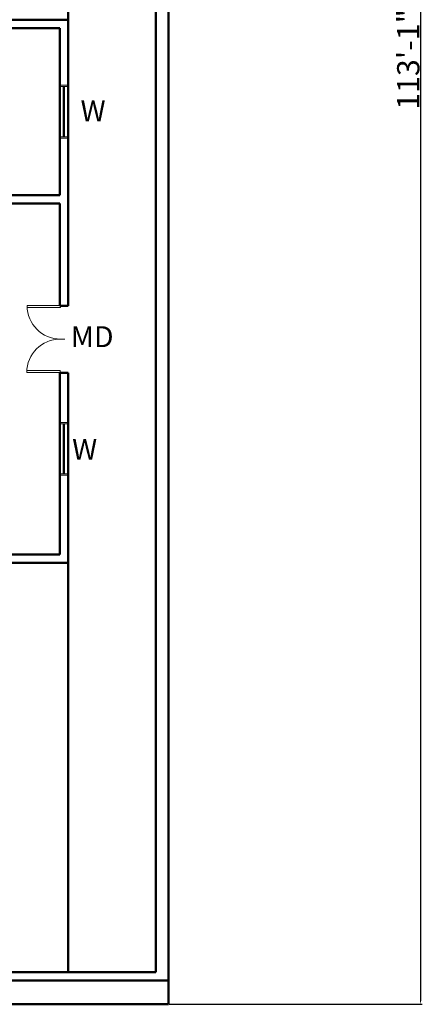
# Model space of a CAD drawing. Units: inches. Extents: x -7040 to -4088, y 6092 to 7645.
# Tile 5 of 11: x -6510 to -6221, y 6157 to 6864. Entities that reach past the tile are written whole.
import ezdxf

# ---------------------------------------------------------------- set-up
doc = ezdxf.new("R2010")
doc.units = ezdxf.units.IN
for name, color, linetype, lineweight in [('A-ANNO-DIMS', 2, 'Continuous', 18), ('A-ANNO-TEXT', 7, 'Continuous', 25), ('A-DOOR', 3, 'Continuous', 18), ('A-GLAZ', 4, 'Continuous', 18), ('A-WALL', 7, 'Continuous', 50)]:
    doc.layers.add(name, color=color, linetype=linetype, lineweight=lineweight)
doc.styles.get("Standard").update_dxf_attribs({"font": 'arial.ttf'})
doc.dimstyles.new('ISO-25', dxfattribs={"dimtxt": 2.5, "dimasz": 2.5, "dimexe": 1.25, "dimexo": 0.625, "dimtad": 1, "dimdec": 0, "dimlunit": 3, "dimtxsty": 'Standard', "dimcen": 2.5, "dimadec": 0, "dimazin": 0, "dimtfac": 1, "dimtdec": 0, "dimtmove": 0, "dimatfit": 3, "dimfxl": 1, "dimarcsym": 0})

# ---------------------------------------------------------------- blocks, each defined once
blk = doc.blocks.new('*U8')
for p, q in [((0, 0), (0, -100)), ((750, 0), (750, -100))]:
    blk.add_line(p, q)
blk.add_lwpolyline([(0, 0), (0, 750), (43.75, 750), (43.75, 0)], close=True)
blk.add_arc((0, 0), 750, 0, 90)
blk = doc.blocks.new('*D93')
at = {"layer": 'A-ANNO-DIMS', "color": 0, "lineweight": -2, "transparency": 16777216}
for p, q in [((-6402.41, 7513.76), (-6220.88, 7513.76)), ((-6222.13, 7511.26), (-6222.13, 6159.26)), ((-6402.41, 6156.76), (-6220.88, 6156.76))]:
    blk.add_line(p, q, dxfattribs=at)
at = {"layer": 'A-ANNO-DIMS', "color": 0, "transparency": 16777216}
for points in [[(-6222.55, 7511.26), (-6221.71, 7511.26), (-6222.13, 7513.76)], [(-6222.55, 6159.26), (-6221.71, 6159.26), (-6222.13, 6156.76)]]:
    blk.add_solid(points, dxfattribs=at)
at = {"layer": 'Defpoints', "color": 0, "transparency": 16777216}
for p in [(-6403.03, 7513.76), (-6403.03, 6156.76), (-6222.13, 6156.76)]:
    blk.add_point(p, dxfattribs=at)
at = {"layer": 'A-ANNO-DIMS', "color": 0, "transparency": 16777216, "insert": (-6230.93, 6835.26), "char_height": 2.5, "attachment_point": 5, "rotation": 90}
blk.add_mtext('{\\H6.4x;113\'-1"}', dxfattribs=at)

msp = doc.modelspace()

# ---------------------------------------------------------------- linework, layer by layer
at = {"layer": 'A-GLAZ'}
for p, q in [((-6481.03, 6816.76), (-6475.03, 6816.76)), ((-6481.03, 6816.76), (-6475.03, 6816.76)), ((-6481.03, 6815.76), (-6475.03, 6815.76)), ((-6481.03, 6815.76), (-6475.03, 6815.76)), ((-6478.53, 6779.76), (-6478.53, 6815.76)), ((-6478.53, 6779.76), (-6478.53, 6815.76)), ((-6478.03, 6779.76), (-6478.03, 6815.76)), ((-6478.03, 6779.76), (-6478.03, 6815.76)), ((-6477.53, 6779.76), (-6477.53, 6815.76)), ((-6477.53, 6779.76), (-6477.53, 6815.76)), ((-6481.03, 6779.76), (-6475.03, 6779.76)), ((-6481.03, 6779.76), (-6475.03, 6779.76)), ((-6481.03, 6778.76), (-6475.03, 6778.76)), ((-6481.03, 6778.76), (-6475.03, 6778.76)), ((-6481.03, 6574.62), (-6475.03, 6574.62)), ((-6481.03, 6574.62), (-6475.03, 6574.62)), ((-6481.03, 6573.62), (-6475.03, 6573.62)), ((-6481.03, 6573.62), (-6475.03, 6573.62)), ((-6478.53, 6537.62), (-6478.53, 6573.62)), ((-6478.53, 6537.62), (-6478.53, 6573.62)), ((-6478.03, 6537.62), (-6478.03, 6573.62)), ((-6478.03, 6537.62), (-6478.03, 6573.62)), ((-6477.53, 6537.62), (-6477.53, 6573.62)), ((-6477.53, 6537.62), (-6477.53, 6573.62)), ((-6481.03, 6537.62), (-6475.03, 6537.62)), ((-6481.03, 6537.62), (-6475.03, 6537.62)), ((-6481.03, 6536.62), (-6475.03, 6536.62)), ((-6481.03, 6536.62), (-6475.03, 6536.62))]:
    msp.add_line(p, q, dxfattribs=at)
at = {"layer": 'A-WALL'}
for p, q in [((-6403.03, 7513.76), (-6403.03, 6156.76)), ((-6412.03, 7504.76), (-6412.03, 6179.76)), ((-6475.03, 7013.76), (-6475.03, 6658.26)), ((-6971.03, 6863.76), (-6475.03, 6863.76)), ((-6641.03, 6857.76), (-6481.03, 6857.76)), ((-6481.03, 6857.76), (-6481.03, 6737.76)), ((-6641.03, 6737.76), (-6481.03, 6737.76)), ((-6773.03, 6731.76), (-6481.03, 6731.76)), ((-6481.03, 6731.76), (-6481.03, 6658.26)), ((-6481.03, 6658.26), (-6475.03, 6658.26)), ((-6481.03, 6610.26), (-6475.03, 6610.26)), ((-6481.03, 6610.26), (-6481.03, 6479.76)), ((-6475.03, 6610.26), (-6475.03, 6179.76)), ((-6773.03, 6479.76), (-6481.03, 6479.76)), ((-6977.03, 6473.76), (-6475.03, 6473.76)), ((-6994.03, 6179.76), (-6412.03, 6179.76)), ((-7003.03, 6173.76), (-6403.03, 6173.76)), ((-7003.03, 6156.76), (-6403.03, 6156.76))]:
    msp.add_line(p, q, dxfattribs=at)

# ---------------------------------------------------------------- block references
at = {"layer": 'A-DOOR'}
for p, xscale, yscale, zscale, rotation in [((-6480.42, 6658.42), -0.0319999999999999, 0.0319999999999999, 0.0319999999999999, 90), ((-6480.6, 6610.41), 0.0319965751455487, 0.0319965751455487, 0.0319965751455487, 90.00000000000003)]:
    msp.add_blockref('*U8', p, dxfattribs=dict(at, xscale=xscale, yscale=yscale, zscale=zscale, rotation=rotation))

# ---------------------------------------------------------------- texts
at = {"layer": 'A-ANNO-TEXT', "char_height": 15, "attachment_point": 1}
for s, insert in [('{W}', (-6466.05, 6805.8)), ('{MD}', (-6473.05, 6643.63)), ('{W}', (-6472.09, 6562.77))]:
    msp.add_mtext_dynamic_manual_height_columns(s, width=701.5203, gutter_width=12.5, heights=[0], dxfattribs=dict(at, insert=insert))

# ---------------------------------------------------------------- dimensions: what is measured, and where the dimension line sits
at = {"layer": 'A-ANNO-DIMS'}
dim = msp.add_linear_dim(base=(-6222.13, 6156.76), p1=(-6403.03, 7513.76), p2=(-6403.03, 6156.76), angle=90, text='{\\H6.4x;<>}', dimstyle='ISO-25', override={"dimclrd": 0, "dimclre": 0, "dimclrt": 0}, dxfattribs=at)
dim.commit()
dim.dimension.update_dxf_attribs({"geometry": '*D93', "text_midpoint": (-6230.93, 6835.26)})

doc.saveas('drawing.dxf')
